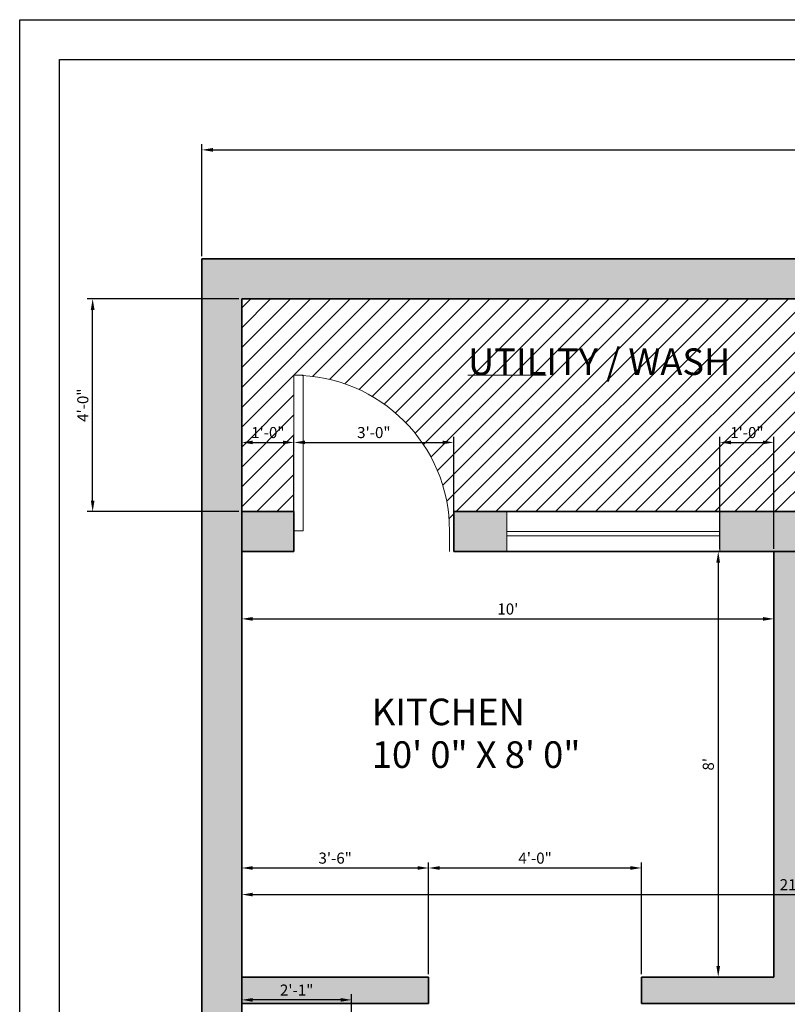
# Model space of a CAD drawing. Units: inches. Extents: x 2998 to 3448, y 1620 to 2377.
# Tile 4 of 5: x 2998 to 3171, y 2155 to 2377. Entities that reach past the tile are written whole.
import ezdxf

# ---------------------------------------------------------------- set-up
doc = ezdxf.new("R2010")
doc.units = ezdxf.units.IN
doc.layers.get('Defpoints').update_dxf_attribs({"color": 110})
for name, color, linetype, lineweight in [('A-ANNO-DIMS', 2, 'Continuous', 18), ('A-ANNO-TTLB', 7, 'Continuous', 25), ('A-AREA-IDEN', 130, 'Continuous', 18), ('A-DOOR', 3, 'Continuous', 18), ('A-FLOR-PATT', 18, 'Continuous', 13), ('A-GLAZ', 4, 'Continuous', 18), ('A-WALL-PATT', 18, 'Continuous', 13), ('C-PROP', 7, 'Continuous', 35), ('L-HRDS-PATT', 175, 'Continuous', 13), ('WALL', 7, 'Continuous', 35)]:
    doc.layers.add(name, color=color, linetype=linetype, lineweight=lineweight)
doc.styles.get("Standard").update_dxf_attribs({"font": 'arial.ttf'})
doc.dimstyles.new('Copy of ISO-25', dxfattribs={"dimtxt": 2.5, "dimasz": 2.5, "dimexe": 1.25, "dimexo": 0.625, "dimtad": 1, "dimdec": 1, "dimlunit": 4, "dimtxsty": 'Standard', "dimcen": 2.5, "dimadec": 0, "dimazin": 0, "dimtfac": 1, "dimtdec": 1, "dimtmove": 0, "dimatfit": 3, "dimfxl": 1, "dimarcsym": 0})

# ---------------------------------------------------------------- blocks, each defined once
blk = doc.blocks.new('*U2')
for p, q in [((0, 0), (0, -100)), ((750, 0), (750, -100))]:
    blk.add_line(p, q)
blk.add_lwpolyline([(0, 0), (0, 750), (43.75, 750), (43.75, 0)], close=True)
blk.add_arc((0, 0), 750, 0, 90)
blk = doc.blocks.new('*D6')
at = {"layer": 'A-ANNO-DIMS', "color": 0, "lineweight": -2, "transparency": 16777216}
for p, q in [((3048.12, 2256.15), (3048.12, 2240.32)), ((3168.12, 2256.15), (3168.12, 2240.32)), ((3050.62, 2241.57), (3165.62, 2241.57))]:
    blk.add_line(p, q, dxfattribs=at)
at = {"layer": 'A-ANNO-DIMS', "color": 0, "transparency": 16777216}
for points in [[(3050.62, 2241.98), (3050.62, 2241.15), (3048.12, 2241.57)], [(3165.62, 2241.98), (3165.62, 2241.15), (3168.12, 2241.57)]]:
    blk.add_solid(points, dxfattribs=at)
at = {"layer": 'Defpoints', "color": 0, "transparency": 16777216}
for p in [(3048.12, 2256.77), (3168.12, 2256.77), (3168.12, 2241.57)]:
    blk.add_point(p, dxfattribs=at)
at = {"layer": 'A-ANNO-DIMS', "color": 0, "transparency": 16777216, "insert": (3108.12, 2243.47), "char_height": 2.5, "attachment_point": 5}
blk.add_mtext("10'", dxfattribs=at)
blk = doc.blocks.new('*D7')
at = {"layer": 'A-ANNO-DIMS', "color": 0, "lineweight": -2, "transparency": 16777216}
for p, q in [((3167.49, 2256.77), (3154.3, 2256.77)), ((3155.55, 2254.27), (3155.55, 2163.27)), ((3167.49, 2160.77), (3154.3, 2160.77))]:
    blk.add_line(p, q, dxfattribs=at)
at = {"layer": 'A-ANNO-DIMS', "color": 0, "transparency": 16777216}
for points in [[(3155.13, 2254.27), (3155.96, 2254.27), (3155.55, 2256.77)], [(3155.13, 2163.27), (3155.96, 2163.27), (3155.55, 2160.77)]]:
    blk.add_solid(points, dxfattribs=at)
at = {"layer": 'Defpoints', "color": 0, "transparency": 16777216}
for p in [(3168.12, 2256.77), (3155.55, 2160.77), (3168.12, 2160.77)]:
    blk.add_point(p, dxfattribs=at)
at = {"layer": 'A-ANNO-DIMS', "color": 0, "transparency": 16777216, "insert": (3153.64, 2208.77), "char_height": 2.5, "attachment_point": 5, "rotation": 90}
blk.add_mtext("8'", dxfattribs=at)
blk = doc.blocks.new('WIN-48IN')
for p, q in [((0, 0), (0, 9)), ((0, 9), (48, 9)), ((48, 9), (48, 0)), ((0, 4.5), (48, 4.5)), ((0, 3.5), (48, 3.5))]:
    blk.add_line(p, q)
blk = doc.blocks.new('*D38')
at = {"layer": 'A-ANNO-DIMS', "color": 0, "lineweight": -2, "transparency": 16777216}
for p, q in [((3048.12, 2144.97), (3048.12, 2156.87)), ((3072.9, 2144.97), (3072.9, 2156.87)), ((3070.4, 2155.62), (3050.62, 2155.62))]:
    blk.add_line(p, q, dxfattribs=at)
at = {"layer": 'A-ANNO-DIMS', "color": 0, "transparency": 16777216}
for points in [[(3050.62, 2156.03), (3050.62, 2155.2), (3048.12, 2155.62)], [(3070.4, 2156.03), (3070.4, 2155.2), (3072.9, 2155.62)]]:
    blk.add_solid(points, dxfattribs=at)
at = {"layer": 'Defpoints', "color": 0}
for p in [(3048.12, 2155.62), (3048.12, 2144.34), (3072.9, 2144.34)]:
    blk.add_point(p, dxfattribs=at)
at = {"layer": 'A-ANNO-DIMS', "color": 0, "transparency": 16777216, "insert": (3060.51, 2157.5), "char_height": 2.5, "attachment_point": 5}
blk.add_mtext('2\'-1"', dxfattribs=at)
blk = doc.blocks.new('*D39')
at = {"layer": 'A-ANNO-DIMS', "color": 0, "lineweight": -2, "transparency": 16777216}
for p, q in [((3039.12, 2323.4), (3039.12, 2348.62)), ((3399.12, 2323.4), (3399.12, 2348.62)), ((3041.62, 2347.37), (3396.62, 2347.37))]:
    blk.add_line(p, q, dxfattribs=at)
at = {"layer": 'A-ANNO-DIMS', "color": 0, "transparency": 16777216}
for points in [[(3041.62, 2347.79), (3041.62, 2346.96), (3039.12, 2347.37)], [(3396.62, 2347.79), (3396.62, 2346.96), (3399.12, 2347.37)]]:
    blk.add_solid(points, dxfattribs=at)
at = {"layer": 'Defpoints', "color": 0}
for p in [(3399.12, 2347.37), (3039.12, 2322.77), (3399.12, 2322.77)]:
    blk.add_point(p, dxfattribs=at)
at = {"layer": 'A-ANNO-DIMS', "color": 0, "transparency": 16777216, "insert": (3219.12, 2349.27), "char_height": 2.5, "attachment_point": 5}
blk.add_mtext('30\'-0"', dxfattribs=at)
blk = doc.blocks.new('*D41')
at = {"layer": 'A-ANNO-DIMS', "color": 0, "lineweight": -2, "transparency": 16777216}
for p, q in [((3047.49, 2313.77), (3013.27, 2313.77)), ((3014.52, 2268.27), (3014.52, 2311.27)), ((3047.49, 2265.77), (3013.27, 2265.77))]:
    blk.add_line(p, q, dxfattribs=at)
at = {"layer": 'A-ANNO-DIMS', "color": 0, "transparency": 16777216}
for points in [[(3014.1, 2311.27), (3014.94, 2311.27), (3014.52, 2313.77)], [(3014.1, 2268.27), (3014.94, 2268.27), (3014.52, 2265.77)]]:
    blk.add_solid(points, dxfattribs=at)
at = {"layer": 'Defpoints', "color": 0}
for p in [(3014.52, 2313.77), (3048.12, 2313.77), (3048.12, 2265.77)]:
    blk.add_point(p, dxfattribs=at)
at = {"layer": 'A-ANNO-DIMS', "color": 0, "transparency": 16777216, "insert": (3012.62, 2289.77), "char_height": 2.5, "attachment_point": 5, "rotation": 90}
blk.add_mtext('4\'-0"', dxfattribs=at)
blk = doc.blocks.new('*D46')
at = {"layer": 'A-ANNO-DIMS', "color": 0, "lineweight": -2, "transparency": 16777216}
for p, q in [((3048.12, 2161.4), (3048.12, 2186.62)), ((3090.26, 2161.4), (3090.26, 2186.62)), ((3050.62, 2185.37), (3087.76, 2185.37))]:
    blk.add_line(p, q, dxfattribs=at)
at = {"layer": 'A-ANNO-DIMS', "color": 0, "transparency": 16777216}
for points in [[(3050.62, 2185.79), (3050.62, 2184.96), (3048.12, 2185.37)], [(3087.76, 2185.79), (3087.76, 2184.96), (3090.26, 2185.37)]]:
    blk.add_solid(points, dxfattribs=at)
at = {"layer": 'Defpoints', "color": 0}
for p in [(3090.26, 2185.37), (3048.12, 2160.77), (3090.26, 2160.77)]:
    blk.add_point(p, dxfattribs=at)
at = {"layer": 'A-ANNO-DIMS', "color": 0, "transparency": 16777216, "insert": (3069.19, 2187.27), "char_height": 2.5, "attachment_point": 5}
blk.add_mtext('3\'-6"', dxfattribs=at)
blk = doc.blocks.new('*D47')
at = {"layer": 'A-ANNO-DIMS', "color": 0, "lineweight": -2, "transparency": 16777216}
for p, q in [((3090.26, 2161.4), (3090.26, 2186.62)), ((3138.26, 2161.4), (3138.26, 2186.62)), ((3092.76, 2185.37), (3135.76, 2185.37))]:
    blk.add_line(p, q, dxfattribs=at)
at = {"layer": 'A-ANNO-DIMS', "color": 0, "transparency": 16777216}
for points in [[(3092.76, 2185.79), (3092.76, 2184.96), (3090.26, 2185.37)], [(3135.76, 2185.79), (3135.76, 2184.96), (3138.26, 2185.37)]]:
    blk.add_solid(points, dxfattribs=at)
at = {"layer": 'Defpoints', "color": 0}
for p in [(3138.26, 2185.37), (3090.26, 2160.77), (3138.26, 2160.77)]:
    blk.add_point(p, dxfattribs=at)
at = {"layer": 'A-ANNO-DIMS', "color": 0, "transparency": 16777216, "insert": (3114.26, 2187.27), "char_height": 2.5, "attachment_point": 5}
blk.add_mtext('4\'-0"', dxfattribs=at)
blk = doc.blocks.new('*D48')
at = {"layer": 'A-ANNO-DIMS', "color": 0, "lineweight": -2, "transparency": 16777216}
for p, q in [((3059.91, 2257.4), (3059.91, 2282.62)), ((3062.41, 2281.37), (3093.41, 2281.37)), ((3095.91, 2257.4), (3095.91, 2282.62))]:
    blk.add_line(p, q, dxfattribs=at)
at = {"layer": 'A-ANNO-DIMS', "color": 0, "transparency": 16777216}
for points in [[(3062.41, 2281.79), (3062.41, 2280.96), (3059.91, 2281.37)], [(3093.41, 2281.79), (3093.41, 2280.96), (3095.91, 2281.37)]]:
    blk.add_solid(points, dxfattribs=at)
at = {"layer": 'Defpoints', "color": 0}
for p in [(3095.91, 2281.37), (3059.91, 2256.77), (3095.91, 2256.77)]:
    blk.add_point(p, dxfattribs=at)
at = {"layer": 'A-ANNO-DIMS', "color": 0, "transparency": 16777216, "insert": (3077.91, 2283.27), "char_height": 2.5, "attachment_point": 5}
blk.add_mtext('3\'-0"', dxfattribs=at)
blk = doc.blocks.new('*D49')
at = {"layer": 'A-ANNO-DIMS', "color": 0, "lineweight": -2, "transparency": 16777216}
for p, q in [((3048.12, 2257.4), (3048.12, 2282.62)), ((3050.62, 2281.37), (3057.41, 2281.37)), ((3059.91, 2257.4), (3059.91, 2282.62))]:
    blk.add_line(p, q, dxfattribs=at)
at = {"layer": 'A-ANNO-DIMS', "color": 0, "transparency": 16777216}
for points in [[(3050.62, 2281.79), (3050.62, 2280.96), (3048.12, 2281.37)], [(3057.41, 2281.79), (3057.41, 2280.96), (3059.91, 2281.37)]]:
    blk.add_solid(points, dxfattribs=at)
at = {"layer": 'Defpoints', "color": 0}
for p in [(3059.91, 2281.37), (3048.12, 2256.77), (3059.91, 2256.77)]:
    blk.add_point(p, dxfattribs=at)
at = {"layer": 'A-ANNO-DIMS', "color": 0, "transparency": 16777216, "insert": (3054.01, 2283.27), "char_height": 2.5, "attachment_point": 5}
blk.add_mtext('1\'-0"', dxfattribs=at)
blk = doc.blocks.new('*D50')
at = {"layer": 'A-ANNO-DIMS', "color": 0, "lineweight": -2, "transparency": 16777216}
for p, q in [((3155.91, 2257.4), (3155.91, 2282.62)), ((3158.41, 2281.37), (3165.62, 2281.37)), ((3168.12, 2257.4), (3168.12, 2282.62))]:
    blk.add_line(p, q, dxfattribs=at)
at = {"layer": 'A-ANNO-DIMS', "color": 0, "transparency": 16777216}
for points in [[(3158.41, 2281.79), (3158.41, 2280.96), (3155.91, 2281.37)], [(3165.62, 2281.79), (3165.62, 2280.96), (3168.12, 2281.37)]]:
    blk.add_solid(points, dxfattribs=at)
at = {"layer": 'Defpoints', "color": 0}
for p in [(3168.12, 2281.37), (3155.91, 2256.77), (3168.12, 2256.77)]:
    blk.add_point(p, dxfattribs=at)
at = {"layer": 'A-ANNO-DIMS', "color": 0, "transparency": 16777216, "insert": (3162.01, 2283.27), "char_height": 2.5, "attachment_point": 5}
blk.add_mtext('1\'-0"', dxfattribs=at)
blk = doc.blocks.new('*D60')
at = {"layer": 'A-ANNO-DIMS', "color": 0, "lineweight": -2, "transparency": 16777216}
for p, q in [((3048.12, 2155.4), (3048.12, 2180.62)), ((3050.62, 2179.37), (3297.62, 2179.37)), ((3300.12, 2155.4), (3300.12, 2180.62))]:
    blk.add_line(p, q, dxfattribs=at)
at = {"layer": 'A-ANNO-DIMS', "color": 0, "transparency": 16777216}
for points in [[(3050.62, 2179.79), (3050.62, 2178.96), (3048.12, 2179.37)], [(3297.62, 2179.79), (3297.62, 2178.96), (3300.12, 2179.37)]]:
    blk.add_solid(points, dxfattribs=at)
at = {"layer": 'Defpoints', "color": 0}
for p in [(3300.12, 2179.37), (3048.12, 2154.77), (3300.12, 2154.77)]:
    blk.add_point(p, dxfattribs=at)
at = {"layer": 'A-ANNO-DIMS', "color": 0, "transparency": 16777216, "insert": (3174.12, 2181.27), "char_height": 2.5, "attachment_point": 5}
blk.add_mtext('21\'-0"', dxfattribs=at)

msp = doc.modelspace()

# ---------------------------------------------------------------- hatches: boundary and pattern name
at = {"layer": 'A-FLOR-PATT'}
h = msp.add_hatch(dxfattribs=at)
h.set_pattern_fill('ANSI31', color=256)
h.paths.add_polyline_path([(3264.12, 1950.77), (3252.12, 1950.77), (3252.12, 1955.56), (3250.03, 1955.56), (3250.03, 1991.39, 0.39722), (3216.23, 1955.56), (3216.23, 1950.77), (3204.12, 1950.77), (3204.12, 1890.77), (3216.12, 1890.77), (3216.12, 1881.77), (3252.12, 1881.77), (3252.12, 1890.77), (3264.12, 1890.77)])
h.paths.add_polyline_path([(3343.37, 2313.77), (3048.12, 2313.77), (3048.12, 2265.77), (3059.91, 2265.77), (3059.91, 2296.51), (3061.95, 2296.51), (3061.95, 2296.45, -0.39722), (3094.97, 2261.45), (3095.91, 2265.77), (3343.37, 2265.77)])
h.paths.add_polyline_path([(3220.44, 1918.61), (3261.55, 1918.61), (3261.55, 1927.8), (3220.44, 1927.8)], flags=24)
h.paths.add_polyline_path([(3220.42, 1928.23), (3252.4, 1928.23), (3252.4, 1937.54), (3220.42, 1937.54)], flags=24)
h.paths.add_polyline_path([(3097.58, 2294.93), (3164.02, 2294.93), (3164.02, 2304.23), (3097.58, 2304.23)], flags=24)
at = {"layer": 'A-WALL-PATT'}
h = msp.add_hatch(color=256, dxfattribs=at)
h.dxf.hatch_style = 1
h.paths.add_polyline_path([(3399.12, 2322.77), (3039.12, 2322.77), (3039.12, 2132.57), (3048.12, 2132.57), (3048.12, 2154.77), (3048.12, 2313.77), (3390.12, 2313.77), (3390.12, 2227.86), (3399.12, 2227.86)])
h.paths.add_polyline_path([(3048.12, 2072.57), (3039.12, 2072.57), (3039.12, 2041.4), (3048.12, 2041.4)])
h.paths.add_polyline_path([(3399.12, 1997.2), (3390.12, 1997.2), (3390.12, 1851.77), (3274.41, 1851.77), (3274.41, 1842.77), (3399.12, 1842.77)])
h.paths.add_polyline_path([(3195.35, 1851.77), (3048.12, 1851.77), (3048.12, 1857.27), (3048.05, 1858.06), (3047.68, 1858.02), (3047.44, 1857.61), (3047.47, 1857.28), (3047.17, 1857.15), (3047.68, 1858.02), (3045.29, 1857.73), (3045.29, 1842.77), (3195.35, 1842.77)])
h.paths.add_polyline_path([(3399.12, 2167.86), (3390.12, 2167.86), (3390.12, 2112.77), (3390.12, 2103.77), (3390.12, 2045.2), (3399.12, 2045.2)])
h.paths.add_polyline_path([(3390.12, 2112.77), (3306.12, 2112.77), (3306.12, 2118.77), (3304.88, 2118.77), (3300.12, 2118.77), (3300.12, 2112.77), (3300.12, 2103.77), (3390.12, 2103.77)])
h.paths.add_polyline_path([(3257.48, 2265.77), (3214.13, 2265.77), (3214.13, 2256.77), (3257.48, 2256.77)], flags=17)
h.paths.add_polyline_path([(3325.36, 2265.77), (3281.48, 2265.77), (3281.48, 2256.77), (3300.12, 2256.77), (3325.36, 2256.77)], flags=17)
h.paths.add_polyline_path([(3390.12, 2265.77), (3373.36, 2265.77), (3373.36, 2256.77), (3390.12, 2256.77)], flags=17)
h.paths.add_polyline_path([(3190.13, 2265.77), (3155.91, 2265.77), (3155.91, 2256.77), (3190.13, 2256.77)], flags=17)
h.paths.add_polyline_path([(3306.12, 2256.77), (3300.12, 2256.77), (3300.12, 2160.77), (3298.12, 2160.77), (3298.12, 2154.77), (3300.12, 2154.77), (3306.12, 2154.77)], flags=17)
h.paths.add_polyline_path([(3240.12, 2256.77), (3234.12, 2256.77), (3234.12, 2160.77), (3215.01, 2160.77), (3215.01, 2154.77), (3268.12, 2154.77), (3268.12, 2158.71), (3268.12, 2160.77), (3240.12, 2160.77)], flags=17)
h.paths.add_polyline_path([(3174.12, 2256.77), (3168.12, 2256.77), (3168.12, 2160.77), (3138.26, 2160.77), (3138.26, 2154.77), (3174.12, 2154.77), (3185.01, 2154.77), (3185.01, 2158.71), (3185.01, 2160.77), (3174.12, 2160.77)], flags=17)
h.paths.add_polyline_path([(3090.26, 2160.77), (3048.12, 2160.77), (3048.12, 2154.77), (3090.26, 2154.77)], flags=17)
h.paths.add_polyline_path([(3072.12, 2058.77), (3048.12, 2058.77), (3048.12, 2049.77), (3072.12, 2049.77)])
h.paths.add_polyline_path([(3298.3, 1959.77), (3270.12, 1959.77), (3270.12, 2061.77), (3300.12, 2061.77), (3306.12, 2061.77), (3306.12, 2067.77), (3300.12, 2067.77), (3264.12, 2067.77), (3264.12, 2061.77), (3264.12, 1959.77), (3252.12, 1959.77), (3252.12, 1955.56), (3252.12, 1950.77), (3264.12, 1950.77), (3264.12, 1890.77), (3264.12, 1881.77), (3273.12, 1881.77), (3273.12, 1950.77), (3298.3, 1950.77)])
h.paths.add_polyline_path([(3390.12, 1959.77), (3358.3, 1959.77), (3358.3, 1950.77), (3390.12, 1950.77)], flags=17)
h.paths.add_polyline_path([(3216.12, 1959.77), (3154.02, 1959.77), (3154.02, 1950.77), (3216.12, 1950.77)])
h.paths.add_polyline_path([(3204.12, 1950.77), (3195.12, 1950.77), (3195.12, 1890.77), (3195.12, 1881.77), (3216.12, 1881.77), (3216.12, 1890.77), (3204.12, 1890.77)])
h.paths.add_polyline_path([(3094.02, 1959.77), (3048.12, 1959.77), (3048.12, 1950.77), (3094.02, 1950.77)])
h.paths.add_polyline_path([(3045.29, 1981.4), (3040.45, 1981.4), (3040.45, 1842.77), (3045.29, 1842.77), (3045.29, 1857.73)])
h.paths.add_polyline_path([(3059.91, 2261.45), (3059.91, 2265.77), (3048.12, 2265.77), (3048.12, 2256.77), (3059.91, 2256.77)], flags=17)
h.paths.add_polyline_path([(3107.91, 2265.77), (3095.91, 2265.77), (3095.91, 2256.77), (3107.91, 2256.77)], flags=17)
h.paths.add_polyline_path([(3274.41, 1851.77), (3264.12, 1851.77), (3264.12, 1846.71), (3264.12, 1842.77), (3274.41, 1842.77)])
h.paths.add_polyline_path([(3204.35, 1851.77), (3195.35, 1851.77), (3195.35, 1842.77), (3204.35, 1842.77), (3204.35, 1846.71)])
at = {"layer": 'L-HRDS-PATT'}
h = msp.add_hatch(dxfattribs=at)
h.set_pattern_fill('_USER', color=256, pattern_type=0)
h.set_pattern_definition([(0, (0, 0), (0, 1), [])])
h.paths.add_polyline_path([(3195.12, 1950.77), (3154.02, 1950.77), (3154.02, 1914.77), (3084.12, 1914.77), (3084.12, 1881.77), (3195.12, 1881.77), (3195.12, 1890.77)])
h.paths.add_polyline_path([(3107.62, 2003.86), (3160.38, 2003.86), (3160.38, 2013.05), (3107.62, 2013.05)], flags=9)
h.paths.add_polyline_path([(3107.6, 2013.48), (3161.48, 2013.48), (3161.48, 2022.79), (3107.6, 2022.79)], flags=9)
h.paths.add_polyline_path([(3162.21, 2109.19), (3212.64, 2109.19), (3212.64, 2118.38), (3162.21, 2118.38)], flags=9)
h.paths.add_polyline_path([(3162.19, 2118.81), (3194.63, 2118.81), (3194.63, 2128.12), (3162.19, 2128.12)], flags=9)
h.paths.add_polyline_path([(3334.58, 2144.47), (3389.67, 2144.47), (3389.67, 2153.66), (3334.58, 2153.66)], flags=9)
h.paths.add_polyline_path([(3334.56, 2154.09), (3390.29, 2154.09), (3390.29, 2163.4), (3334.56, 2163.4)], flags=9)
h.paths.add_polyline_path([(3245.01, 2216.14), (3288.45, 2216.14), (3288.45, 2225.33), (3245.01, 2225.33)], flags=9)
h.paths.add_polyline_path([(3244.99, 2225.76), (3277.44, 2225.76), (3277.44, 2235.07), (3244.99, 2235.07)], flags=9)
h.paths.add_polyline_path([(3181.61, 2212.67), (3207.44, 2212.67), (3207.44, 2221.86), (3181.61, 2221.86)], flags=9)
h.paths.add_polyline_path([(3181.59, 2222.28), (3214.03, 2222.28), (3214.03, 2231.6), (3181.59, 2231.6)], flags=9)
h.paths.add_polyline_path([(3075.92, 2206.31), (3126.35, 2206.31), (3126.35, 2215.5), (3075.92, 2215.5)], flags=9)
h.paths.add_polyline_path([(3075.9, 2215.93), (3115.79, 2215.93), (3115.79, 2225.24), (3075.9, 2225.24)], flags=9)
h.paths.add_polyline_path([(3097.58, 2294.93), (3164.02, 2294.93), (3164.02, 2304.23), (3097.58, 2304.23)], flags=9)
h = msp.add_hatch(dxfattribs=at)
h.set_pattern_fill('ANGLE', color=256)
h.set_pattern_definition([(0, (0, 0), (0, 6.985), [5.08, -1.905]), (90, (0, 0), (-6.985, 4e-16), [5.08, -1.905])])
h.paths.add_polyline_path([(3390.12, 1950.77), (3358.3, 1950.77), (3273.12, 1950.77), (3273.12, 1881.77), (3268.62, 1881.77), (3268.62, 1851.77), (3390.12, 1851.77)])
h.paths.add_polyline_path([(3334.58, 2144.47), (3389.67, 2144.47), (3389.67, 2153.66), (3334.58, 2153.66)], flags=9)
h.paths.add_polyline_path([(3334.56, 2154.09), (3390.29, 2154.09), (3390.29, 2163.4), (3334.56, 2163.4)], flags=9)
h.paths.add_polyline_path([(3220.44, 1918.61), (3261.55, 1918.61), (3261.55, 1927.8), (3220.44, 1927.8)], flags=9)
h.paths.add_polyline_path([(3220.42, 1928.23), (3252.4, 1928.23), (3252.4, 1937.54), (3220.42, 1937.54)], flags=9)
h.paths.add_polyline_path([(3220.62, 1853.01), (3246.55, 1853.01), (3246.55, 1862.32), (3220.62, 1862.32)], flags=9)
h.paths.add_polyline_path([(3084.85, 1856.81), (3130.62, 1856.81), (3130.62, 1866), (3084.85, 1866)], flags=9)
h.paths.add_polyline_path([(3084.83, 1866.42), (3123.8, 1866.42), (3123.8, 1875.73), (3084.83, 1875.73)], flags=9)
h.paths.add_polyline_path([(3297.1, 1896.73), (3349.87, 1896.73), (3349.87, 1905.92), (3297.1, 1905.92)], flags=24)
h.paths.add_polyline_path([(3297.08, 1906.35), (3357.94, 1906.35), (3357.94, 1915.66), (3297.08, 1915.66)], flags=24)
h.paths.add_polyline_path([(3107.62, 2003.86), (3160.38, 2003.86), (3160.38, 2013.05), (3107.62, 2013.05)], flags=9)
h.paths.add_polyline_path([(3107.6, 2013.48), (3161.48, 2013.48), (3161.48, 2022.79), (3107.6, 2022.79)], flags=9)
h.paths.add_polyline_path([(3294.47, 2015.87), (3347.23, 2015.87), (3347.23, 2025.06), (3294.47, 2025.06)], flags=9)
h.paths.add_polyline_path([(3294.45, 2025.49), (3350.19, 2025.49), (3350.19, 2034.8), (3294.45, 2034.8)], flags=9)
h.paths.add_polyline_path([(3162.21, 2109.19), (3212.64, 2109.19), (3212.64, 2118.38), (3162.21, 2118.38)], flags=9)
h.paths.add_polyline_path([(3162.19, 2118.81), (3194.63, 2118.81), (3194.63, 2128.12), (3162.19, 2128.12)], flags=9)
h.paths.add_polyline_path([(3075.92, 2206.31), (3126.35, 2206.31), (3126.35, 2215.5), (3075.92, 2215.5)], flags=9)
h.paths.add_polyline_path([(3075.9, 2215.93), (3115.79, 2215.93), (3115.79, 2225.24), (3075.9, 2225.24)], flags=9)

# ---------------------------------------------------------------- linework, layer by layer
at = {"layer": 'A-ANNO-TTLB'}
for points in [[(2998.07, 2376.74), (3447.79, 2376.74), (3447.79, 1619.66), (2998.07, 1619.66)], [(3007.07, 2367.74), (3438.79, 2367.74), (3438.79, 1628.66), (3007.07, 1628.66)]]:
    msp.add_lwpolyline(points, close=True, dxfattribs=at)
at = {"layer": 'A-AREA-IDEN'}
msp.add_line((3099.13, 2296.58), (3116.75, 2296.58), dxfattribs=at)
at = {"layer": 'C-PROP'}
for points in [[(3039.12, 2322.77), (3399.12, 2322.77), (3399.12, 1842.77), (3039.12, 1842.77)], [(3048.12, 2313.77), (3390.12, 2313.77), (3390.12, 1851.77), (3048.12, 1851.77)]]:
    msp.add_lwpolyline(points, close=True, dxfattribs=at)
at = {"layer": 'WALL'}
for p, q in [((3048.12, 2313.77), (3048.12, 2265.77)), ((3048.12, 2265.77), (3059.91, 2265.77)), ((3059.91, 2256.77), (3059.91, 2265.77)), ((3095.91, 2265.77), (3095.91, 2256.77)), ((3095.91, 2265.77), (3390.12, 2265.77)), ((3048.12, 2256.77), (3048.12, 2160.77)), ((3059.91, 2256.77), (3048.12, 2256.77)), ((3390.12, 2256.77), (3095.91, 2256.77)), ((3095.91, 2256.77), (3107.91, 2256.77)), ((3168.12, 2160.77), (3168.12, 2256.77)), ((3168.12, 2256.77), (3174.12, 2256.77)), ((3048.12, 2160.77), (3090.26, 2160.77)), ((3090.26, 2154.77), (3090.26, 2160.77)), ((3168.12, 2160.77), (3138.26, 2160.77)), ((3138.26, 2160.77), (3138.26, 2154.77)), ((3138.26, 2160.77), (3168.12, 2160.77)), ((3048.12, 2154.77), (3048.12, 2058.77)), ((3090.26, 2154.77), (3048.12, 2154.77)), ((3174.12, 2154.77), (3138.26, 2154.77))]:
    msp.add_line(p, q, dxfattribs=at)

# ---------------------------------------------------------------- block references
at = {"layer": 'A-DOOR', "xscale": 0.0467476429000655, "yscale": 0.0467476429000655, "zscale": 0.0467476429000655}
msp.add_blockref('*U2', (3059.91, 2261.45), dxfattribs=at)
at = {"layer": 'A-GLAZ'}
msp.add_blockref('WIN-48IN', (3107.91, 2256.77), dxfattribs=at)

# ---------------------------------------------------------------- texts
at = {"layer": 'A-AREA-IDEN'}
for s, p in [('UTILITY / WASH', (3099.13, 2296.58)), ('KITCHEN', (3077.45, 2217.58)), ('10\' 0" X 8\' 0"', (3077.45, 2207.95))]:
    msp.add_text(s, height=6, dxfattribs=at).set_placement(p)

# ---------------------------------------------------------------- dimensions: what is measured, and where the dimension line sits
at = {"layer": 'A-ANNO-DIMS'}
for base, p1, p2, override, picture, middle in [((3399.12, 2347.37), (3039.12, 2322.77), (3399.12, 2322.77), {"dimdec": 1, "dimlfac": 1, "dimrnd": 0, "dimzin": 1, "dimdsep": 46, "dimlunit": 4, "dimfrac": 2}, '*D39', (3219.12, 2349.27)), ((3059.91, 2281.37), (3048.12, 2256.77), (3059.91, 2256.77), {"dimdec": 1, "dimlfac": 1, "dimrnd": 0, "dimzin": 1, "dimdsep": 46, "dimlunit": 4, "dimfrac": 2}, '*D49', (3054.01, 2283.27)), ((3168.12, 2281.37), (3155.91, 2256.77), (3168.12, 2256.77), {"dimdec": 1, "dimlfac": 1, "dimrnd": 0, "dimzin": 1, "dimdsep": 46, "dimlunit": 4, "dimfrac": 2}, '*D50', (3162.01, 2283.27)), ((3168.12, 2241.57), (3048.12, 2256.77), (3168.12, 2256.77), {"dimclrd": 0, "dimclre": 0, "dimclrt": 0}, '*D6', (3108.12, 2243.47)), ((3090.26, 2185.37), (3048.12, 2160.77), (3090.26, 2160.77), {"dimdec": 1, "dimlfac": 1, "dimrnd": 0, "dimzin": 1, "dimdsep": 46, "dimlunit": 4, "dimfrac": 2}, '*D46', (3069.19, 2187.27)), ((3138.26, 2185.37), (3090.26, 2160.77), (3138.26, 2160.77), {"dimdec": 1, "dimlfac": 1, "dimrnd": 0, "dimzin": 1, "dimdsep": 46, "dimlunit": 4, "dimfrac": 2}, '*D47', (3114.26, 2187.27))]:
    dim = msp.add_linear_dim(base=base, p1=p1, p2=p2, dimstyle='Copy of ISO-25', override=override, dxfattribs=at)
    dim.commit()
    dim.dimension.update_dxf_attribs({"geometry": picture, "text_midpoint": middle})
for base, p1, p2, angle, override, picture, middle in [((3014.52, 2313.77), (3048.12, 2265.77), (3048.12, 2313.77), 90, {"dimdec": 1, "dimlfac": 1, "dimrnd": 0, "dimzin": 1, "dimdsep": 46, "dimlunit": 4, "dimfrac": 2}, '*D41', (3012.62, 2289.77)), ((3095.91, 2281.37), (3059.91, 2256.77), (3095.91, 2256.77), 0, {"dimdec": 1, "dimlfac": 1, "dimrnd": 0, "dimzin": 1, "dimdsep": 46, "dimlunit": 4, "dimfrac": 2}, '*D48', (3077.91, 2283.27)), ((3155.55, 2160.77), (3168.12, 2256.77), (3168.12, 2160.77), 90, {"dimclrd": 0, "dimclre": 0, "dimclrt": 0}, '*D7', (3153.64, 2208.77)), ((3300.12, 2179.37), (3048.12, 2154.77), (3300.12, 2154.77), 0, {"dimdec": 1, "dimlfac": 1, "dimrnd": 0, "dimzin": 1, "dimdsep": 46, "dimlunit": 4, "dimfrac": 2}, '*D60', (3174.12, 2181.27)), ((3048.12, 2155.62), (3072.9, 2144.34), (3048.12, 2144.34), 180, {"dimdec": 1, "dimlfac": 1, "dimrnd": 0, "dimzin": 1, "dimdsep": 46, "dimlunit": 4, "dimfrac": 2}, '*D38', (3060.51, 2157.5))]:
    dim = msp.add_linear_dim(base=base, p1=p1, p2=p2, angle=angle, dimstyle='Copy of ISO-25', override=override, dxfattribs=at)
    dim.commit()
    dim.dimension.update_dxf_attribs({"geometry": picture, "text_midpoint": middle})

doc.saveas('drawing.dxf')
